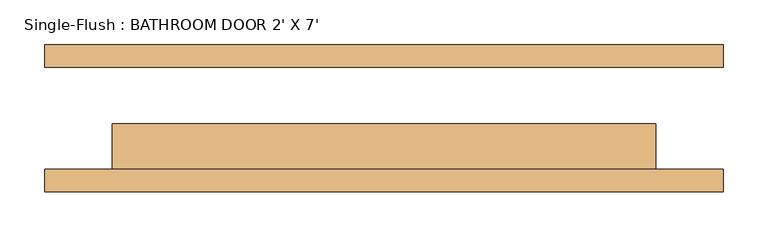
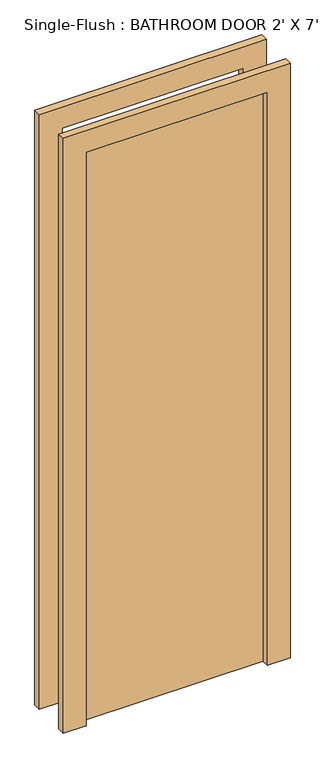
"""IFC4 building model written with IfcOpenShell, lengths in millimetres: door geometry, Single-Flush : BATHROOM DOOR 2' X 7'."""

from ifc_helpers import new_model, si_unit, frame, origin, origin_with_axes, place, context, project, spatial, polyline, outline, extrude, source, transform, mapped, element, save


def single_flush_bathroom_door_2_x_7_e2285e44(model_context):
    return source(origin(), model_context, "Body", "SweptSolid", [
        extrude(outline(polyline([(2108.2, -381.0), (0.0, -381.0), (0.0, -304.8), (2032.0, -304.8), (2032.0, 304.8), (0.0, 304.8), (0.0, 381.0), (2108.2, 381.0), (2108.2, -381.0)])), frame((0.0, -82.55, 0.0), z_axis=(0.0, 1.0, 0.0), x_axis=(0.0, 0.0, 1.0)), (0.0, 0.0, 1.0), 25.4),
        extrude(outline(polyline([(2108.2, 381.0), (2108.2, -381.0), (0.0, -381.0), (0.0, -304.8), (2032.0, -304.8), (2032.0, 304.8), (0.0, 304.8), (0.0, 381.0), (2108.2, 381.0)])), frame((0.0, 57.15, 0.0), z_axis=(0.0, 1.0, 0.0), x_axis=(0.0, 0.0, 1.0)), (0.0, 0.0, 1.0), 25.4),
        extrude(outline(polyline([(304.8, -6.35), (304.8, -57.15), (-304.8, -57.15), (-304.8, -6.35), (304.8, -6.35)])), origin_with_axes(), (0.0, 0.0, 1.0), 2032.0),
    ])


if __name__ == "__main__":
    model = new_model("IFC4")
    model_context = context("Model", 3, world=origin())
    ifc_project = project(units=[si_unit("LENGTHUNIT", "METRE", prefix="MILLI")], contexts=[model_context])
    site = spatial("IfcSite", under=ifc_project)
    building = spatial("IfcBuilding", under=site)
    placement = place(None, origin())
    single_flush_bathroom_door_2_x_7_shape = single_flush_bathroom_door_2_x_7_e2285e44(model_context)
    element("IfcDoor", 1, ObjectType="Single-Flush : BATHROOM DOOR 2' X 7'", at=placement, inside=building, context=model_context, shape_type="MappedRepresentation", body=[
        mapped(single_flush_bathroom_door_2_x_7_shape, transform((0.0, 0.0, 0.0), x_axis=(1.0, 0.0, 0.0), y_axis=(0.0, 1.0, 0.0), z_axis=(0.0, 0.0, 1.0))),
    ])
    save(model, "model.ifc")

# Revit data of these elements
# Type "Single-Flush : BATHROOM DOOR 2' X 7'"
#   Type Mark = "11"
#   Construction Type Id = "MDOOR"
#   Assembly Code = "C1020"
#   Analytic Construction = "Metal"
#   Thickness = 0' - 2"
#   Heat Transfer Coefficient (U) = 0.651978 BTU/(h·ft²·°F)
#   Height = 6' - 8"
#   Trim Projection Ext = 0' - 1"
#   Trim Projection Int = 0' - 1"
#   Trim Width = 0' - 3"
#   Width = 2' - 0"
#   Define Thermal Properties by = 1
#   Door Material = Door - Panel
#   Frame Material = Door - Frame
#   Visual Light Transmittance = 0
#   Solar Heat Gain Coefficient = 0
#   Function = (empty or 0)
#   Wall Closure = (empty or 0)
# Element 1 (IfcDoor, "Single-Flush : BATHROOM DOOR 2' X 7'")
#   Materials on its faces: "Door - Frame", "Door - Panel"
# Materials
#   "Door - Panel": class "Wood", colour RGB 210 159 95, transparency 0, Cost = 0
#   "Door - Frame": colour RGB 118 70 51, transparency 0, Cost = 0
